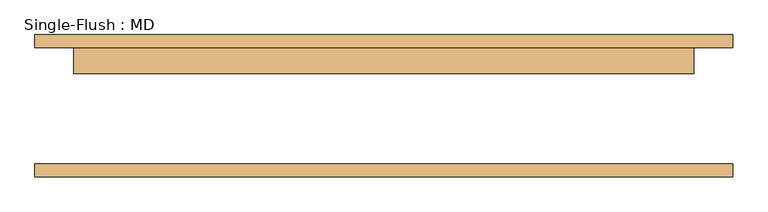
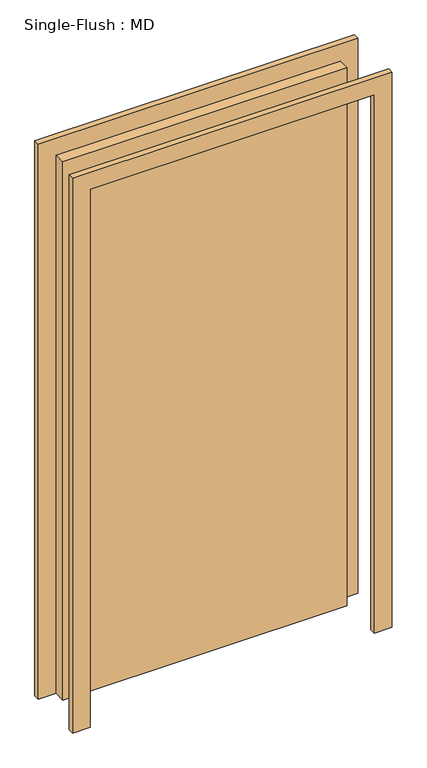
"""IFC4 building model written with IfcOpenShell, lengths in millimetres: door geometry, Single-Flush : MD."""

from ifc_helpers import new_model, si_unit, frame, origin, origin_with_axes, place, context, project, spatial, polyline, outline, extrude, source, transform, mapped, element, save


def single_flush_md_e3fbe821(model_context):
    return source(origin(), model_context, "Body", "SweptSolid", [
        extrude(outline(polyline([(2514.6, -685.8), (0.0, -685.8), (0.0, -609.6), (2438.4, -609.6), (2438.4, 609.6), (0.0, 609.6), (0.0, 685.8), (2514.6, 685.8), (2514.6, -685.8)])), frame((0.0, 114.3, 0.0), z_axis=(0.0, 1.0, 0.0), x_axis=(0.0, 0.0, 1.0)), (0.0, 0.0, 1.0), 25.4),
        extrude(outline(polyline([(2514.6, 685.8), (2514.6, -685.8), (0.0, -685.8), (0.0, -609.6), (2438.4, -609.6), (2438.4, 609.6), (0.0, 609.6), (0.0, 685.8), (2514.6, 685.8)])), frame((0.0, -139.7, 0.0), z_axis=(0.0, 1.0, 0.0), x_axis=(0.0, 0.0, 1.0)), (0.0, 0.0, 1.0), 25.4),
        extrude(outline(polyline([(609.6, 63.5), (-609.6, 63.5), (-609.6, 114.3), (609.6, 114.3), (609.6, 63.5)])), origin_with_axes(), (0.0, 0.0, 1.0), 2438.4),
    ])


if __name__ == "__main__":
    model = new_model("IFC4")
    model_context = context("Model", 3, world=origin())
    ifc_project = project(units=[si_unit("LENGTHUNIT", "METRE", prefix="MILLI")], contexts=[model_context])
    site = spatial("IfcSite", under=ifc_project)
    building = spatial("IfcBuilding", under=site)
    placement = place(None, origin())
    single_flush_md_shape = single_flush_md_e3fbe821(model_context)
    element("IfcDoor", 1, ObjectType="Single-Flush : MD", at=placement, inside=building, context=model_context, shape_type="MappedRepresentation", body=[
        mapped(single_flush_md_shape, transform((0.0, 0.0, 0.0), x_axis=(1.0, 0.0, 0.0), y_axis=(0.0, 1.0, 0.0), z_axis=(0.0, 0.0, 1.0))),
    ])
    save(model, "model.ifc")

# Revit data of these elements
# Type "Single-Flush : MD"
#   Type Mark = "10"
#   Construction Type Id = "MDOOR"
#   Assembly Code = "C1020"
#   Analytic Construction = "Metal"
#   Thickness = 0' - 2"
#   Heat Transfer Coefficient (U) = 0.651978 BTU/(h·ft²·°F)
#   Height = 8' - 0"
#   Trim Projection Ext = 0' - 1"
#   Trim Projection Int = 0' - 1"
#   Trim Width = 0' - 3"
#   Width = 4' - 0"
#   Define Thermal Properties by = 1
#   Door Material = Door - Panel
#   Frame Material = Door - Frame
#   Visual Light Transmittance = 0
#   Solar Heat Gain Coefficient = 0
#   Function = (empty or 0)
#   Wall Closure = (empty or 0)
# Element 1 (IfcDoor, "Single-Flush : MD")
#   Materials on its faces: "Door - Frame", "Door - Panel"
# Materials
#   "Door - Panel": class "Wood", colour RGB 210 159 95, transparency 0, Cost = 0
#   "Door - Frame": colour RGB 118 70 51, transparency 0, Cost = 0
